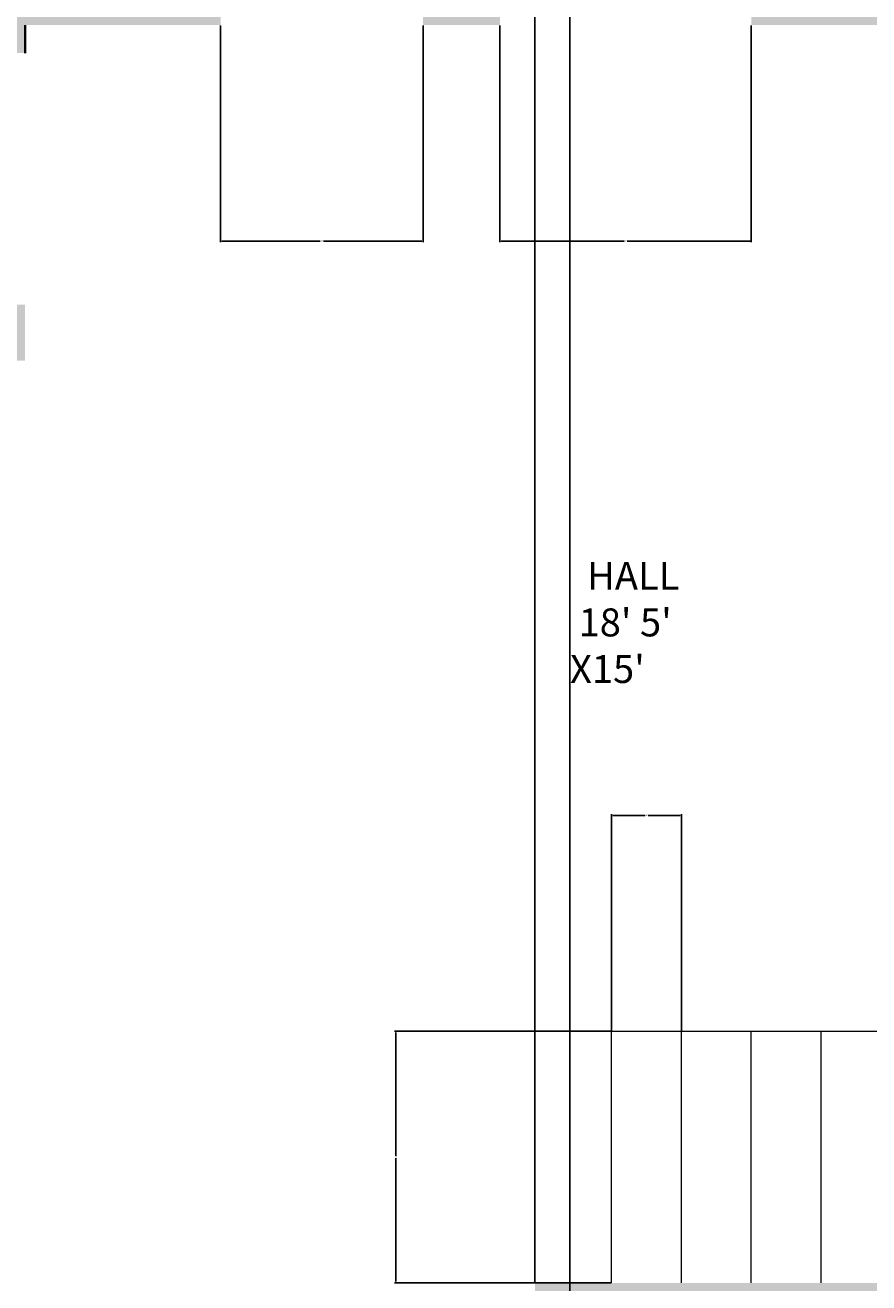
# Model space of a CAD drawing. Units: inches. Extents: x -30 to 437, y -29 to 647.
# Tile 10 of 15: x 187 to 308, y 255 to 435. Entities that reach past the tile are written whole.
import ezdxf

# ---------------------------------------------------------------- set-up
doc = ezdxf.new("R2010")
doc.units = ezdxf.units.IN
doc.header["$MEASUREMENT"] = 0
for name, color, linetype, lineweight in [('A-ANNO-DIMS', 2, 'Continuous', 18), ('A-AREA-IDEN', 7, 'Continuous', 18), ('A-FLOR-STRS', 7, 'Continuous', 18), ('A-WALL', 7, 'Continuous', 35)]:
    doc.layers.add(name, color=color, linetype=linetype, lineweight=lineweight)
doc.layers.add('A-WALL-PATT', color=251, linetype='Continuous', lineweight=13, true_color=0x636466)
doc.styles.get("Standard").update_dxf_attribs({"font": 'arial.ttf'})
doc.dimstyles.get("Standard").update_dxf_attribs({"dimtxt": 0.18, "dimasz": 0.18, "dimexe": 0.18, "dimexo": 0.0625, "dimgap": 0.09, "dimtad": 0, "dimtih": 1, "dimtoh": 1, "dimdec": 4, "dimzin": 0, "dimdsep": 46, "dimtxsty": 'Standard', "dimcen": 0.09, "dimadec": 0, "dimazin": 0, "dimtfac": 1, "dimtdec": 4, "dimtofl": 0, "dimtmove": 0, "dimatfit": 3, "dimfxl": 1, "dimtolj": 1, "dimtzin": 0, "dimarcsym": 0})

# ---------------------------------------------------------------- blocks, each defined once
blk = doc.blocks.new('*D43')
at = {"layer": 'A-ANNO-DIMS', "color": 0, "lineweight": -2, "transparency": 16777216}
for p, q in [((214.67, 434.48), (214.67, 403.47)), ((243.67, 434.48), (243.67, 403.47)), ((214.85, 403.65), (228.95, 403.65)), ((243.49, 403.65), (229.39, 403.65))]:
    blk.add_line(p, q, dxfattribs=at)
at = {"layer": 'A-ANNO-DIMS', "color": 0, "transparency": 16777216}
for points in [[(214.85, 403.68), (214.85, 403.62), (214.67, 403.65)], [(243.49, 403.68), (243.49, 403.62), (243.67, 403.65)]]:
    blk.add_solid(points, dxfattribs=at)
at = {"layer": 'Defpoints', "color": 0, "transparency": 16777216}
for p in [(214.67, 434.55), (243.67, 434.55), (214.67, 403.65)]:
    blk.add_point(p, dxfattribs=at)
at = {"layer": 'A-ANNO-DIMS', "color": 0, "transparency": 16777216, "insert": (229.17, 403.65), "char_height": 0.18, "attachment_point": 5}
blk.add_mtext('\\A1;29', dxfattribs=at)
blk = doc.blocks.new('*D44')
at = {"layer": 'A-ANNO-DIMS', "color": 0, "lineweight": -2, "transparency": 16777216}
for p, q in [((254.67, 434.48), (254.67, 403.47)), ((290.67, 434.48), (290.67, 403.47)), ((254.85, 403.65), (272.45, 403.65)), ((290.49, 403.65), (272.89, 403.65))]:
    blk.add_line(p, q, dxfattribs=at)
at = {"layer": 'A-ANNO-DIMS', "color": 0, "transparency": 16777216}
for points in [[(254.85, 403.68), (254.85, 403.62), (254.67, 403.65)], [(290.49, 403.68), (290.49, 403.62), (290.67, 403.65)]]:
    blk.add_solid(points, dxfattribs=at)
at = {"layer": 'Defpoints', "color": 0, "transparency": 16777216}
for p in [(254.67, 434.55), (290.67, 434.55), (254.67, 403.65)]:
    blk.add_point(p, dxfattribs=at)
at = {"layer": 'A-ANNO-DIMS', "color": 0, "transparency": 16777216, "insert": (272.67, 403.65), "char_height": 0.18, "attachment_point": 5}
blk.add_mtext('\\A1;36', dxfattribs=at)
blk = doc.blocks.new('*D45')
at = {"layer": 'A-ANNO-DIMS', "color": 0, "lineweight": -2, "transparency": 16777216}
for p, q in [((270.61, 290.55), (239.59, 290.55)), ((239.77, 290.37), (239.77, 272.73)), ((239.77, 254.73), (239.77, 272.37)), ((270.61, 254.55), (239.59, 254.55))]:
    blk.add_line(p, q, dxfattribs=at)
at = {"layer": 'A-ANNO-DIMS', "color": 0, "transparency": 16777216}
for points in [[(239.74, 290.37), (239.8, 290.37), (239.77, 290.55)], [(239.74, 254.73), (239.8, 254.73), (239.77, 254.55)]]:
    blk.add_solid(points, dxfattribs=at)
at = {"layer": 'Defpoints', "color": 0, "transparency": 16777216}
for p in [(239.77, 290.55), (270.67, 290.55), (270.67, 254.55)]:
    blk.add_point(p, dxfattribs=at)
at = {"layer": 'A-ANNO-DIMS', "color": 0, "transparency": 16777216, "insert": (239.77, 272.55), "char_height": 0.18, "attachment_point": 5}
blk.add_mtext('\\A1;36', dxfattribs=at)
blk = doc.blocks.new('*D46')
at = {"layer": 'A-ANNO-DIMS', "color": 0, "lineweight": -2, "transparency": 16777216}
for p, q in [((270.67, 290.61), (270.67, 321.63)), ((270.85, 321.45), (275.46, 321.45)), ((280.49, 321.45), (275.88, 321.45)), ((280.67, 290.61), (280.67, 321.63))]:
    blk.add_line(p, q, dxfattribs=at)
at = {"layer": 'A-ANNO-DIMS', "color": 0, "transparency": 16777216}
for points in [[(270.85, 321.48), (270.85, 321.42), (270.67, 321.45)], [(280.49, 321.48), (280.49, 321.42), (280.67, 321.45)]]:
    blk.add_solid(points, dxfattribs=at)
at = {"layer": 'Defpoints', "color": 0, "transparency": 16777216}
for p in [(280.67, 321.45), (270.67, 290.55), (280.67, 290.55)]:
    blk.add_point(p, dxfattribs=at)
at = {"layer": 'A-ANNO-DIMS', "color": 0, "transparency": 16777216, "insert": (275.67, 321.45), "char_height": 0.18, "attachment_point": 5}
blk.add_mtext('\\A1;10', dxfattribs=at)
blk = doc.blocks.new('*D54')
at = {"layer": 'A-ANNO-DIMS', "color": 0, "lineweight": -2, "transparency": 16777216}
for p, q in [((259.67, 254.61), (259.67, 646.63)), ((259.85, 646.45), (262.02, 646.45)), ((264.49, 646.45), (262.32, 646.45)), ((264.67, 249.61), (264.67, 646.63))]:
    blk.add_line(p, q, dxfattribs=at)
at = {"layer": 'A-ANNO-DIMS', "color": 0, "transparency": 16777216}
for points in [[(259.85, 646.48), (259.85, 646.42), (259.67, 646.45)], [(264.49, 646.48), (264.49, 646.42), (264.67, 646.45)]]:
    blk.add_solid(points, dxfattribs=at)
at = {"layer": 'Defpoints', "color": 0, "transparency": 16777216}
for p in [(259.67, 646.45), (259.67, 254.55), (264.67, 249.55)]:
    blk.add_point(p, dxfattribs=at)
at = {"layer": 'A-ANNO-DIMS', "color": 0, "transparency": 16777216, "insert": (262.17, 646.45), "char_height": 0.18, "attachment_point": 5}
blk.add_mtext('\\A1;5', dxfattribs=at)

msp = doc.modelspace()

# ---------------------------------------------------------------- hatches: boundary and pattern name
at = {"layer": 'A-WALL-PATT'}
h = msp.add_hatch(color=256, dxfattribs=at)
h.dxf.hatch_style = 1
h.paths.add_polyline_path([(393.6054, 183.2352), (369.6054, 183.2352), (369.6054, 213.2352), (393.6054, 213.2352), (393.6054, 207.2352), (394.6054, 207.2352), (394.6054, 211.2352), (395.6054, 211.2352), (395.6054, 185.2352), (394.6054, 185.2352), (394.6054, 189.2352), (393.6054, 189.2352)], flags=0)
h.paths.add_polyline_path([(384.6054, 189.2352, -1), (390.6054, 189.2352, -1)], flags=0)
h.paths.add_polyline_path([(385.6054, 189.2352, -1), (389.6054, 189.2352, -1)], flags=0)
h.paths.add_polyline_path([(374.6054, 189.2352, -1), (382.6054, 189.2352, -1)], flags=0)
h.paths.add_polyline_path([(386.6054, 189.2352, -1), (388.6054, 189.2352, -1)], flags=0)
h.paths.add_polyline_path([(375.6054, 189.2352, -1), (381.6054, 189.2352, -1)], flags=0)
h.paths.add_polyline_path([(376.6054, 189.2352, -1), (380.6054, 189.2352, -1)], flags=0)
h.paths.add_polyline_path([(377.6054, 189.2352, -1), (379.6054, 189.2352, -1)], flags=0)
h.paths.add_polyline_path([(390.6054, 195.2352), (374.6054, 195.2352), (374.6054, 201.2352), (390.6054, 201.2352)], flags=0)
h.paths.add_polyline_path([(389.6054, 196.2352), (375.6054, 196.2352), (375.6054, 200.2352), (389.6054, 200.2352)], flags=0)
h.paths.add_polyline_path([(383.6054, 207.2352, -1), (391.6054, 207.2352, -1)], flags=0)
h.paths.add_polyline_path([(384.6054, 207.2352, -1), (390.6054, 207.2352, -1)], flags=0)
h.paths.add_polyline_path([(385.6054, 207.2352, -1), (389.6054, 207.2352, -1)], flags=0)
h.paths.add_polyline_path([(386.6054, 207.2352, -1), (388.6054, 207.2352, -1)], flags=0)
h.paths.add_polyline_path([(375.6054, 207.2352, -1), (381.6054, 207.2352, -1)], flags=0)
h.paths.add_polyline_path([(376.6054, 207.2352, -1), (380.6054, 207.2352, -1)], flags=0)
h.paths.add_polyline_path([(377.6054, 207.2352, -1), (379.6054, 207.2352, -1)], flags=0)
h.paths.add_polyline_path([(305.5437, 160.3663, -0.41421356), (304.0437, 158.8663), (271.0437, 158.8663, -0.41421356), (269.5437, 160.3663), (269.5437, 178.3663, -0.41421356), (271.0437, 179.8663), (304.0437, 179.8663, -0.41421356), (305.5437, 178.3663)], flags=0)
h.paths.add_polyline_path([(304.0437, 165.3663, -0.41421356), (303.0437, 164.3663), (289.2937, 164.3663, -0.41421356), (288.2937, 165.3663), (288.2937, 177.3663, -0.41421356), (289.2937, 178.3663), (303.0437, 178.3663, -0.41421356), (304.0437, 177.3663)], flags=0)
h.paths.add_polyline_path([(296.5437, 171.3663, -1), (295.5437, 171.3663, -1)], flags=0)
h.paths.add_polyline_path([(286.7937, 165.3663, -0.41421356), (285.7937, 164.3663), (272.0437, 164.3663, -0.41421356), (271.0437, 165.3663), (271.0437, 177.3663, -0.41421356), (272.0437, 178.3663), (285.7937, 178.3663, -0.41421356), (286.7937, 177.3663)], flags=0)
h.paths.add_polyline_path([(279.5437, 171.3663, -1), (278.5437, 171.3663, -1)], flags=0)
h.paths.add_polyline_path([(360.6737, 290.5474), (360.6737, 300.5474), (396.6737, 300.5474), (396.6737, 290.5474)], flags=0)
h.paths.add_polyline_path([(259.6737, 124.5474), (259.6737, 114.5474), (171.6737, 114.5474), (171.6737, 124.5474)], flags=0)
h.paths.add_polyline_path([(288.0737, 215.3705), (286.7097, 214.583), (268.7097, 245.7599), (270.0737, 246.5474)], flags=0)
h.paths.add_polyline_path([(259.6737, 168.5474), (256.6737, 168.5474), (256.6737, 173.5474), (256.6737, 179.0224), (255.8753, 177.6395), (224.2956, 195.872, 0.12053744), (220.1737, 179.0224, 0.12053744), (216.0518, 195.872), (184.4721, 177.6395), (183.6737, 179.0224), (215.2836, 197.2724), (216.0821, 195.8895), (216.0518, 195.872, -0.12053744), (220.1737, 179.0224, -0.12053744), (224.2956, 195.872), (224.2653, 195.8895), (225.0638, 197.2724), (256.6737, 179.0224), (256.6737, 173.5474), (259.6737, 173.5474)], flags=0)
h.paths.add_polyline_path([(386.7943, 325.4601), (372.6871, 325.4601), (372.6871, 339.5673), (386.7943, 339.5673)], flags=0)
h.paths.add_polyline_path([(359.5875, 343.7429), (357.7905, 343.7429), (357.7905, 327.9179), (359.3933, 327.9179, 0.41420885), (361.5302, 330.0549), (361.5302, 341.8434, 0.41436161)], flags=0)
h.paths.add_polyline_path([(341.7887, 323.1235, -0.11921667), (340.7839, 323.1235)], flags=0)
h.paths.add_polyline_path([(379.6332, 328.8632), (379.6332, 332.2699), (376.0992, 332.2699, 0.39427733)], flags=0)
h.paths.add_polyline_path([(375.5299, 332.459, -1), (383.8511, 332.459, -1)], flags=0)
h.paths.add_polyline_path([(388.9363, 344.7425), (372.5309, 344.7425, -0.41421356), (370.394, 346.8794), (370.394, 347.5594, -0.39085173), (372.3472, 349.7005, -0.43951011), (370.394, 351.4933), (370.394, 365.1894, -0.40305452), (372.2191, 367.1298, -0.41839453), (370.394, 368.9291), (370.394, 382.6251, -0.40885826), (372.2519, 384.5722, -0.42377324), (370.394, 386.3707), (370.394, 400.0667, -0.38660687), (372.1327, 402.0094), (372.531, 402.0094, -0.41421834), (370.394, 404.1464), (370.394, 404.7778, -0.41420891), (372.5309, 406.9147), (388.9363, 406.9147, -0.41421821), (391.0733, 404.7778), (391.0733, 346.8794, -0.41421356)], flags=0)
edge = h.paths.add_edge_path(flags=0)
edge.add_spline(control_points=[(349.3585, 363.204), (349.0859, 363.204), (348.8133, 363.2227), (348.2712, 363.2973), (348.0016, 363.3531), (347.3533, 363.5328), (346.9776, 363.6755), (346.2445, 364.0308), (345.887, 364.2432), (345.1953, 364.7329), (344.8611, 365.0101), (344.2197, 365.6237), (343.9125, 365.9603), (343.211, 366.8336), (342.8313, 367.3965), (342.1401, 368.6117), (341.8286, 369.2641), (341.2807, 370.64), (341.0443, 371.3636), (340.6522, 372.8619), (340.4964, 373.6367), (340.2695, 375.2158), (340.1983, 376.0203), (340.142, 377.6365), (340.157, 378.4483), (340.2729, 380.0567), (340.3738, 380.8533), (340.6589, 382.4093), (340.8432, 383.1686), (341.2906, 384.629), (341.5538, 385.3301), (342.1531, 386.6544), (342.4891, 387.2776), (343.2266, 388.4288), (343.6281, 388.9567), (344.4879, 389.9012), (344.9463, 390.3178), (345.7981, 390.9428), (346.182, 391.1771), (346.9712, 391.5648), (347.3766, 391.7182), (348.2004, 391.9387), (348.6189, 392.0058), (349.4588, 392.0508), (349.8801, 392.0288), (350.7146, 391.8966), (351.1278, 391.7865), (351.9366, 391.4822), (352.3323, 391.2882), (353.0989, 390.8223), (353.4699, 390.5504), (354.1819, 389.9355), (354.5229, 389.5924), (355.1706, 388.8418), (355.4772, 388.4343), (356.1315, 387.4422), (356.4671, 386.8397), (357.0692, 385.5581), (357.3356, 384.879), (357.7933, 383.4624), (357.9846, 382.725), (358.2875, 381.2112), (358.3992, 380.4349), (358.5404, 378.8643), (358.5699, 378.0699), (358.546, 376.4841), (358.4926, 375.6928), (358.3042, 374.1343), (358.1692, 373.3672), (357.8207, 371.8774), (357.6072, 371.1549), (357.1067, 369.7735), (356.8196, 369.1148), (356.1782, 367.8787), (355.8238, 367.3013), (355.0551, 366.244), (354.6408, 365.7641), (353.7607, 364.9161), (353.2948, 364.5481), (352.445, 364.0149), (352.0701, 363.822), (351.3034, 363.5117), (350.9116, 363.3943), (350.1325, 363.2418), (349.7455, 363.204), (349.3585, 363.204)], knot_values=[3.14159265, 3.14159265, 3.14159265, 3.14159265, 3.22691715, 3.22691715, 3.31224165, 3.31224165, 3.43426671, 3.43426671, 3.55629177, 3.55629177, 3.67831683, 3.67831683, 3.8003419, 3.8003419, 3.97157384, 3.97157384, 4.14280577, 4.14280577, 4.31403771, 4.31403771, 4.48526965, 4.48526965, 4.65650159, 4.65650159, 4.82773353, 4.82773353, 4.99896547, 4.99896547, 5.1701974, 5.1701974, 5.34142934, 5.34142934, 5.51266128, 5.51266128, 5.68389322, 5.68389322, 5.85512516, 5.85512516, 5.98669107, 5.98669107, 6.11825699, 6.11825699, 6.24982291, 6.24982291, 6.38138882, 6.38138882, 6.51295474, 6.51295474, 6.64452065, 6.64452065, 6.77608657, 6.77608657, 6.90765249, 6.90765249, 7.0392184, 7.0392184, 7.20701563, 7.20701563, 7.37481286, 7.37481286, 7.54261009, 7.54261009, 7.71040732, 7.71040732, 7.87820455, 7.87820455, 8.04600178, 8.04600178, 8.21379901, 8.21379901, 8.38159624, 8.38159624, 8.54939347, 8.54939347, 8.7171907, 8.7171907, 8.88498794, 8.88498794, 9.05278517, 9.05278517, 9.17820699, 9.17820699, 9.30362881, 9.30362881, 9.42477796, 9.42477796, 9.42477796, 9.42477796], degree=3, periodic=0)
edge.add_line((341.1696, 384.3006), (341.2012, 384.2808))
edge = h.paths.add_edge_path(flags=0)
edge.add_line((344.3353, 388.7801), (344.317, 388.7915))
edge.add_ellipse((349.3585, 377.6204), major_axis=(0, -13.7895), ratio=0.62186025, start_angle=-244.867444, end_angle=-124.769923)
h.paths.add_polyline_path([(163.6737, 163.1474), (132.4968, 145.1474), (131.7093, 146.5114), (162.8862, 164.5114)], flags=0)
h.paths.add_polyline_path([(366.4355, 409.0896, -0.41423669), (364.2985, 406.9525, -0.4913499), (361.5302, 408.8973), (361.5302, 420.6405, 0.41421356), (359.3932, 422.7775), (357.7905, 422.7775), (357.7905, 406.9525), (359.6317, 406.9525, 0.42741026), (361.5332, 408.9757, 0.39869469), (363.6672, 406.9525, 0.51958103), (366.4355, 409.0895)], flags=0)
h.paths.add_polyline_path([(386.7943, 410.9671), (372.6871, 410.9671), (372.6871, 425.0742), (386.7943, 425.0742)], flags=0)
h.paths.add_polyline_path([(379.6332, 414.3701), (379.6332, 417.7768), (376.0992, 417.7768, 0.39427733)], flags=0)
h.paths.add_polyline_path([(375.5299, 417.966, -1), (383.8511, 417.966, -1)], flags=0)
h.paths.add_polyline_path([(150.0377, 351.583), (148.6737, 352.3705), (166.6737, 383.5474), (168.0377, 382.7599)], flags=0)
h.paths.add_polyline_path([(91.6737, 234.1974), (66.559, 219.6974), (65.9246, 220.7962), (91.0393, 235.2962)], flags=0)
h.paths.add_polyline_path([(255.4612, 443.5834), (254.6737, 444.9474), (285.8506, 462.9474), (286.6381, 461.5834)], flags=0)
h.paths.add_polyline_path([(176.2737, 394.5474), (158.2737, 425.7243), (159.6377, 426.5118), (177.6377, 395.3349)], flags=0)
h.paths.add_polyline_path([(243.6737, 439.5474), (243.0393, 438.4486), (217.9246, 452.9486), (218.559, 454.0474)], flags=0)
h.paths.add_polyline_path([(38.1264, 269.8429), (40.2408, 269.8429), (40.2408, 270.3508), (38.1264, 270.3508)], flags=0)
h.paths.add_polyline_path([(75.7157, 289.9439), (40.2408, 289.9439), (38.1264, 289.6524), (40.2408, 289.6524)], flags=0)
h.paths.add_polyline_path([(75.7157, 270.0846), (77.6447, 270.0846), (77.6697, 270.1626), (75.7175, 270.1626)], flags=0)
h.paths.add_polyline_path([(80.5373, 293.3002), (33.0467, 293.3002), (13.5054, 293.3002), (13.5054, 351.9244), (29.7898, 351.9244), (80.5373, 351.9244)], flags=0)
h.paths.add_polyline_path([(46.0261, 212.466, -0.50131678), (27.1651, 207.5106), (21.165, 209.5107), (21.165, 206.5107), (22.665, 206.5107), (22.665, 203.5107), (21.165, 203.5107), (21.165, 203.0107), (13.165, 203.0107), (13.165, 224.0107), (21.165, 224.0107), (21.165, 217.5107), (27.1649, 219.5106, -0.50132349), (46.0261, 214.5554, -0.13289091)], flags=0)
h.paths.add_polyline_path([(44.688, 211.8666, -0.48007965), (27.165, 209.5107), (27.165, 217.5107, -0.4800795), (44.688, 215.1547, -0.21500378)], flags=0)
h.paths.add_polyline_path([(19.415, 204.0107), (15.165, 204.0107, -0.41421356), (14.165, 204.7607), (14.165, 222.0107, -0.41421356), (14.915, 223.0107), (19.165, 223.0107, -0.41421356), (20.165, 222.2607), (20.165, 205.0107, -0.41421356)], flags=0)
h.paths.add_polyline_path([(32.7608, 269.0719), (31.8439, 269.0719), (31.8439, 268.6134), (13.5054, 268.6134), (13.5054, 291.5366), (31.8439, 291.5366), (32.7608, 291.0781), (32.7608, 280.9919, -1), (32.7608, 279.1581)], flags=0)
h.paths.add_polyline_path([(40.2408, 360.1436), (38.1264, 360.1436), (38.1264, 359.6357), (40.2408, 359.6357)], flags=0)
h.paths.add_polyline_path([(75.7157, 355.2807), (40.2408, 355.2807), (38.1264, 355.5722), (40.2408, 355.5722), (40.2408, 355.2807), (75.7157, 355.2807), (75.7157, 375.5982), (40.2408, 375.5982), (38.1264, 375.3817), (40.2408, 375.3817), (40.2408, 375.5982), (75.7157, 375.5982), (77.9733, 375.062), (75.7175, 375.062), (75.7175, 374.554)], flags=0)
h.paths.add_polyline_path([(42.8174, 299.814, 0.13867074), (34.1602, 294.603), (14.8081, 294.603), (14.8081, 350.6216), (29.8539, 350.6216, 0.09822056)], flags=0)
h.paths.add_polyline_path([(15.8636, 276.7781, -0.30640166), (20.3757, 283.4499), (20.3483, 290.6726), (31.4014, 290.7146), (31.4309, 282.9124), (26.8287, 282.895, -0.26006276), (30.241, 276.7781, -1)], flags=0)
h.paths.add_polyline_path([(26.1332, 276.7781), (23.0523, 273.6972), (19.9714, 276.7781), (23.0523, 279.8589), (23.0523, 283.9209), (21.3493, 283.9145), (20.7006, 283.5219), (20.6907, 286.1226), (23.2914, 286.1325), (25.8936, 285.7522), (27.1939, 285.7572), (28.4928, 286.1522), (31.0935, 286.1621), (31.0918, 286.6172), (25.6303, 286.5965), (25.616, 290.3675), (31.0775, 290.3882), (31.0918, 286.6172), (31.1034, 283.5614), (28.5027, 283.5515), (25.9005, 283.9317), (23.0523, 283.9209), (23.0523, 279.8589)], flags=0)
h.paths.add_polyline_path([(24.0793, 276.7781, -1), (22.0253, 276.7781, -1)], flags=0)
h.paths.add_polyline_path([(35.7687, 302.2895, -0.41421356), (35.2283, 301.2726), (22.2164, 297.2909, -0.41421356), (21.1995, 297.8313), (15.7317, 315.6996, -0.41421356), (16.2721, 316.7165), (18.8554, 317.507), (15.3721, 328.8904, -0.41421356), (15.9125, 329.9073), (28.9244, 333.889, -0.41421356), (29.9414, 333.3486), (35.4091, 315.4802, -0.41421356), (34.8687, 314.4633), (32.2854, 313.6728)], flags=0)
h.paths.add_polyline_path([(361.3728, 532.6207), (302.7487, 532.6207), (302.7487, 580.1113), (302.7487, 599.6527), (361.3728, 599.6527), (361.3728, 583.3682)], flags=0)
h.paths.add_polyline_path([(370.1, 575.0316), (370.1, 572.9172), (370.6079, 572.9172), (370.6079, 575.0316)], flags=0)
h.paths.add_polyline_path([(385.0466, 537.4423), (385.0466, 572.9172), (384.8302, 575.0316), (384.8302, 572.9172)], flags=0)
h.paths.add_polyline_path([(384.5104, 535.3262), (384.5104, 537.4406), (384.0025, 537.4406), (364.7291, 537.4423), (364.7291, 572.9172), (365.0206, 575.0316), (365.0206, 572.9172), (364.7291, 572.9172), (364.7291, 537.4423), (384.5884, 537.4423), (384.5884, 535.5133)], flags=0)
h.paths.add_polyline_path([(384.5884, 535.5133), (383.4945, 535.164), (383.4945, 537.4406), (382.9866, 535.3262), (382.9866, 537.4406), (383.4945, 535.3262), (383.4945, 537.4406), (384.5884, 537.4406)], flags=0)
h.paths.add_polyline_path([(23.874, 286.8174), (21.0132, 286.8065), (21.0004, 290.1875), (23.8612, 290.1983)], flags=0)
h.paths.add_polyline_path([(242.9824, 511.1667), (234.9824, 511.1667), (234.9824, 517.6667), (228.9825, 515.6667, -0.50132349), (210.1213, 520.622, -0.13289091), (210.1213, 522.7114, -0.50131678), (228.9823, 527.6667), (234.9824, 525.6667), (234.9824, 528.6667), (233.4824, 528.6667), (233.4824, 531.6667), (234.9824, 531.6667), (234.9824, 532.1667), (242.9824, 532.1667)], flags=0)
h.paths.add_polyline_path([(236.9824, 512.1667, -0.41421356), (235.9824, 512.9167), (235.9824, 530.1667, -0.41421356), (236.7324, 531.1667), (240.9824, 531.1667, -0.41421356), (241.9824, 530.4167), (241.9824, 513.1667, -0.41421356), (241.2324, 512.1667)], flags=0)
h.paths.add_polyline_path([(279.533, 537.4423), (279.533, 535.5133), (279.6111, 535.4884), (279.6111, 537.4406)], flags=0)
h.paths.add_polyline_path([(279.2913, 575.0316), (279.2913, 572.9172), (279.7992, 572.9172), (279.7992, 575.0316)], flags=0)
h.paths.add_polyline_path([(211.4594, 520.0227, -0.21500378), (211.4594, 523.3107, -0.48007965), (228.9824, 525.6667), (228.9824, 517.6667, -0.4800795)], flags=0)
h.paths.add_polyline_path([(32.7627, 354.1465), (31.8457, 354.1465), (31.8457, 353.688), (13.5054, 353.688), (13.5054, 376.6134), (31.8457, 376.6134), (32.7627, 376.1549), (32.7627, 366.0677, -1), (32.7627, 364.2337)], flags=0)
h.paths.add_polyline_path([(15.9446, 365.1507, -1), (30.3234, 365.1507, -1)], flags=0)
h.paths.add_polyline_path([(41.213, 428.467), (43.3274, 428.467), (43.3274, 428.9749), (41.213, 428.9749)], flags=0)
h.paths.add_polyline_path([(78.8022, 448.568), (43.3274, 448.568), (41.213, 448.2765), (43.3274, 448.2765)], flags=0)
h.paths.add_polyline_path([(78.8022, 428.7087), (80.7313, 428.7087), (80.7562, 428.7868), (78.804, 428.7868)], flags=0)
h.paths.add_polyline_path([(26.2152, 365.1507), (23.134, 362.0696), (20.0529, 365.1507), (23.134, 368.2319)], flags=0)
h.paths.add_polyline_path([(24.1611, 365.1507, -1), (22.107, 365.1507, -1)], flags=0)
h.paths.add_polyline_path([(309.2625, 570.3406, 0.13867074), (304.0514, 578.9978), (304.0514, 598.3499), (360.07, 598.3499), (360.07, 583.3041, 0.09822056)], flags=0)
h.paths.add_polyline_path([(246.6737, 552.5474), (129.6737, 552.5474), (129.6737, 606.5474), (246.6737, 606.5474)], flags=16)
h.paths.add_polyline_path([(373.6822, 580.3953), (363.595, 580.3953), (363.595, 581.3123), (363.1365, 581.3123), (363.1365, 599.6527), (386.0619, 599.6527), (386.0619, 581.3123), (385.6034, 580.3953), (375.5162, 580.3953, -1)], flags=0)
h.paths.add_polyline_path([(83.6239, 451.9244), (36.1333, 451.9244), (16.5919, 451.9244), (16.5919, 510.5485), (32.8764, 510.5485), (83.6239, 510.5485)], flags=0)
h.paths.add_polyline_path([(367.4098, 590.024, -1), (381.7886, 590.024, -1)], flags=0)
h.paths.add_polyline_path([(374.5992, 586.9428), (371.518, 590.024), (374.5992, 593.1052), (377.6803, 590.024)], flags=0)
h.paths.add_polyline_path([(373.5721, 590.024, -1), (375.6262, 590.024, -1)], flags=0)
h.paths.add_polyline_path([(324.9287, 577.7489, -0.41421356), (323.9118, 578.2893), (323.1212, 580.8726), (311.7379, 577.3893, -0.41421356), (310.721, 577.9297), (306.7393, 590.9416, -0.41421356), (307.2797, 591.9585), (325.1481, 597.4263, -0.41421356), (326.165, 596.8859), (326.9555, 594.3026), (338.3388, 597.7859, -0.41421356), (339.3557, 597.2455), (343.3374, 584.2336, -0.41421356), (342.797, 583.2167)], flags=0)
h.paths.add_polyline_path([(300.5265, 580.3972), (290.4404, 580.3972, -1), (288.6065, 580.3972), (278.5203, 580.3972), (278.5203, 581.3142), (278.0619, 581.3142), (278.0619, 599.6527), (300.985, 599.6527), (300.985, 581.3142)], flags=0)
h.paths.add_polyline_path([(300.163, 581.7567), (292.3609, 581.7271), (292.3434, 586.3294, -0.75567924), (279.0378, 590.1057, -0.82536731), (292.8983, 592.7823), (300.1211, 592.8097)], flags=0)
h.paths.add_polyline_path([(299.8367, 582.0805), (296.0656, 582.0662), (293.0098, 582.0546), (292.9999, 584.6553), (293.3802, 587.2575), (293.3694, 590.1057), (289.3074, 590.1057), (286.2265, 587.0248), (283.1456, 590.1057), (286.2265, 593.1866), (289.3074, 590.1057), (293.3694, 590.1057), (293.3629, 591.8088), (292.9703, 592.4575), (295.5711, 592.4673), (295.5809, 589.8666), (295.2007, 587.2644), (295.2056, 585.9641), (295.6006, 584.6652), (295.6105, 582.0645), (296.0656, 582.0662), (296.0449, 587.5277), (299.8159, 587.542)], flags=0)
h.paths.add_polyline_path([(285.1995, 590.1057, -1), (287.2535, 590.1057, -1)], flags=0)
h.paths.add_polyline_path([(299.6467, 589.2969), (296.2658, 589.284), (296.255, 592.1448), (299.6359, 592.1576)], flags=0)
h.paths.add_polyline_path([(35.8473, 427.696), (34.9304, 427.696), (34.9304, 427.2376), (16.5919, 427.2376), (16.5919, 450.1607), (34.9304, 450.1607), (35.8473, 449.7022), (35.8473, 439.6161, -1), (35.8473, 437.7822)], flags=0)
h.paths.add_polyline_path([(18.9502, 435.4022, -0.30640166), (23.4623, 442.074), (23.4349, 449.2968), (34.4879, 449.3387), (34.5175, 441.5366), (29.9152, 441.5191, -0.26006276), (33.3275, 435.4022, -1)], flags=0)
h.paths.add_polyline_path([(29.2197, 435.4022), (26.1389, 432.3213), (23.058, 435.4022), (26.1389, 438.4831), (26.1389, 442.5451), (24.4358, 442.5386), (23.7871, 442.1461), (23.7772, 444.7468), (26.378, 444.7566), (28.9801, 444.3764), (30.2805, 444.3813), (31.5794, 444.7764), (34.1801, 444.7862), (34.1784, 445.2413), (28.7169, 445.2206), (28.7026, 448.9917), (34.164, 449.0124), (34.1784, 445.2413), (34.1899, 442.1855), (31.5892, 442.1756), (28.987, 442.5559), (26.1389, 442.5451), (26.1389, 438.4831)], flags=0)
h.paths.add_polyline_path([(27.1658, 435.4022, -1), (25.1119, 435.4022, -1)], flags=0)
h.paths.add_polyline_path([(45.904, 458.4382, 0.13867074), (37.2467, 453.2271), (17.8947, 453.2271), (17.8947, 509.2457), (32.9405, 509.2457, 0.09822056)], flags=0)
h.paths.add_polyline_path([(26.9605, 445.4415), (24.0997, 445.4307), (24.0869, 448.8116), (26.9477, 448.8225)], flags=0)
h.paths.add_polyline_path([(38.3149, 459.8967), (25.3029, 455.915, -0.41421356), (24.286, 456.4554), (18.8183, 474.3238, -0.41421356), (19.3586, 475.3407), (21.942, 476.1312), (18.4587, 487.5145, -0.41421356), (18.999, 488.5314), (32.011, 492.5131, -0.41421356), (33.0279, 491.9727), (38.4957, 474.1044, -0.41421356), (37.9553, 473.0875), (35.3719, 472.297), (38.8553, 460.9136, -0.41421356)], flags=0)
h.paths.add_polyline_path([(43.3274, 518.7678), (41.213, 518.7678), (41.213, 518.2598), (43.3274, 518.2598)], flags=0)
h.paths.add_polyline_path([(78.8022, 513.9049), (43.3274, 513.9049), (41.213, 514.1964), (43.3274, 514.1964), (43.3274, 513.9049), (78.8022, 513.9049), (78.8022, 534.2223), (43.3274, 534.2223), (41.213, 534.0059), (43.3274, 534.0059), (43.3274, 534.2223), (78.8022, 534.2223), (81.0599, 533.6861), (78.804, 533.6861), (78.804, 533.1782)], flags=0)
h.paths.add_polyline_path([(121.6737, 556.8974), (121.0393, 555.7986), (95.9246, 570.2986), (96.559, 571.3974)], flags=0)
h.paths.add_polyline_path([(35.8493, 512.7707), (34.9322, 512.7707), (34.9322, 512.3122), (16.5919, 512.3122), (16.5919, 535.2376), (34.9322, 535.2376), (35.8493, 534.7791), (35.8493, 524.6919, -1), (35.8493, 522.8579)], flags=0)
h.paths.add_polyline_path([(19.0312, 523.7749, -1), (33.41, 523.7749, -1)], flags=0)
h.paths.add_polyline_path([(26.2206, 520.6937), (23.1394, 523.7749), (26.2206, 526.8561), (29.3018, 523.7749)], flags=0)
h.paths.add_polyline_path([(25.1935, 523.7749, -1), (27.2476, 523.7749, -1)], flags=0)
h.paths.add_polyline_path([(28.4381, 586.0173), (22.438, 588.0173), (22.438, 585.0173), (23.938, 585.0173), (23.938, 582.0173), (22.438, 582.0173), (22.438, 581.5173), (14.438, 581.5173), (14.438, 602.5173), (22.438, 602.5173), (22.438, 596.0173), (28.4379, 598.0173, -0.50132349), (47.2992, 593.062, -0.13289091), (47.2992, 590.9726, -0.50131678)], flags=0)
h.paths.add_polyline_path([(28.438, 588.0174), (28.438, 596.0173, -0.4800795), (45.961, 593.6614, -0.21500378), (45.961, 590.3733, -0.48007965)], flags=0)
h.paths.add_polyline_path([(20.688, 582.5173), (16.438, 582.5173, -0.41421356), (15.438, 583.2673), (15.438, 600.5173, -0.41421356), (16.188, 601.5173), (20.438, 601.5173, -0.41421356), (21.438, 600.7673), (21.438, 583.5173, -0.41421356)], flags=0)
h.paths.add_polyline_path([(171.6737, 2.0474), (171.6737, 104.5474), (259.6737, 104.5474), (259.6737, 148.5474), (396.6737, 148.5474), (396.6737, 2.0474), (405.6737, 2.0474), (405.6737, 615.5474), (1.6737, 615.5474), (1.6737, 2.0474)])
h.paths.add_polyline_path([(171.6737, 104.5474), (259.6737, 104.5474), (259.6737, 210.5474), (264.6737, 210.5474), (264.6737, 153.5474), (396.6737, 153.5474), (396.6737, 249.5474), (264.6737, 249.5474), (264.6737, 246.5474), (259.6737, 246.5474), (259.6737, 254.5474), (396.6737, 254.5474), (396.6737, 434.5474), (290.6737, 434.5474), (290.6737, 439.5474), (396.6737, 439.5474), (396.6737, 606.5474), (251.6737, 606.5474), (251.6737, 439.5474), (254.6737, 439.5474), (254.6737, 434.5474), (243.6737, 434.5474), (243.6737, 439.5474), (246.6737, 439.5474), (246.6737, 547.5474), (186.6737, 547.5474), (186.6737, 439.5474), (214.6737, 439.5474), (214.6737, 434.5474), (186.6737, 434.5474), (186.6737, 430.5474), (181.6737, 430.5474), (181.6737, 547.5474), (121.6737, 547.5474), (121.6737, 552.5474), (124.6737, 552.5474), (124.6737, 606.5474), (10.6737, 606.5474), (10.6737, 552.5474), (92.6737, 552.5474), (92.6737, 547.5474), (10.6737, 547.5474), (10.6737, 391.5474), (181.6737, 391.5474), (181.6737, 394.5474), (186.6737, 394.5474), (186.6737, 386.5474), (171.6737, 386.5474), (171.6737, 383.5474), (166.6737, 383.5474), (166.6737, 386.5474), (10.6737, 386.5474), (10.6737, 238.5474), (62.6737, 238.5474), (62.6737, 233.5474), (10.6737, 233.5474), (10.6737, 173.5474), (94.6737, 173.5474), (94.6737, 233.5474), (91.6737, 233.5474), (91.6737, 238.5474), (166.6737, 238.5474), (166.6737, 347.5474), (171.6737, 347.5474), (171.6737, 233.5474), (99.6737, 233.5474), (99.6737, 173.5474), (127.6737, 173.5474), (127.6737, 168.5474), (10.6737, 168.5474), (10.6737, 11.0474), (166.6737, 11.0474), (166.6737, 168.5474), (163.6737, 168.5474), (163.6737, 173.5474), (183.6737, 173.5474), (183.6737, 168.5474), (171.6737, 168.5474)])

# ---------------------------------------------------------------- linework, layer by layer
at = {"layer": 'A-FLOR-STRS'}
for p, q in [((270.6737, 254.5474), (270.6737, 290.5474)), ((270.6737, 290.5474), (396.6737, 290.5474)), ((280.6737, 254.5474), (280.6737, 290.5474)), ((290.6737, 254.5474), (290.6737, 290.5474)), ((300.6737, 254.5474), (300.6737, 290.5474))]:
    msp.add_line(p, q, dxfattribs=at)
at = {"layer": 'A-WALL'}
msp.add_line((186.6737, 430.5474), (186.6737, 434.5474), dxfattribs=at)

# ---------------------------------------------------------------- texts
at = {"layer": 'A-AREA-IDEN', "insert": (264.7149, 357.7356), "char_height": 4, "attachment_point": 1}
msp.add_mtext_dynamic_manual_height_columns("  HALL          18' 5' X15' ", width=25.99481, gutter_width=1, heights=[0], dxfattribs=at)

# ---------------------------------------------------------------- dimensions: what is measured, and where the dimension line sits
at = {"layer": 'A-ANNO-DIMS'}
for base, p1, p2, picture, middle in [((259.6737, 646.4474), (264.6737, 249.5474), (259.6737, 254.5474), '*D54', (262.1737, 646.4474)), ((280.6737, 321.4474), (270.6737, 290.5474), (280.6737, 290.5474), '*D46', (275.6737, 321.4474))]:
    dim = msp.add_linear_dim(base=base, p1=p1, p2=p2, dimstyle='Standard', override={"dimdec": 0, "dimlfac": 1, "dimrnd": 0, "dimzin": 0, "dimdsep": 46, "dimlunit": 2}, dxfattribs=at)
    dim.commit()
    dim.dimension.update_dxf_attribs({"geometry": picture, "text_midpoint": middle})
for base, p1, p2, angle, picture, middle in [((214.6737, 403.6474), (243.6737, 434.5474), (214.6737, 434.5474), 180, '*D43', (229.1737, 403.6474)), ((254.6737, 403.6474), (290.6737, 434.5474), (254.6737, 434.5474), 180, '*D44', (272.6737, 403.6474)), ((239.7737, 290.5474), (270.6737, 254.5474), (270.6737, 290.5474), 90, '*D45', (239.7737, 272.5474))]:
    dim = msp.add_linear_dim(base=base, p1=p1, p2=p2, angle=angle, dimstyle='Standard', override={"dimdec": 0, "dimlfac": 1, "dimrnd": 0, "dimzin": 0, "dimdsep": 46, "dimlunit": 2}, dxfattribs=at)
    dim.commit()
    dim.dimension.update_dxf_attribs({"geometry": picture, "text_midpoint": middle})

doc.saveas('drawing.dxf')
